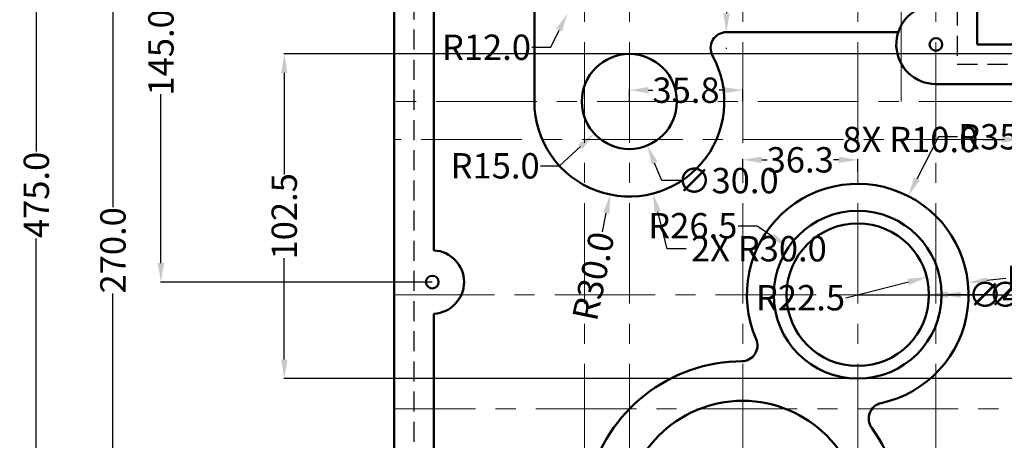
# Model space of a CAD drawing. Units: inches. Extents: x 11765 to 12471, y 10149 to 10793.
# Tile 2 of 8: x 11765 to 12076, y 10397 to 10530. Entities that reach past the tile are written whole.
import ezdxf

# ---------------------------------------------------------------- set-up
doc = ezdxf.new("R2010")
doc.units = ezdxf.units.IN
doc.header["$MEASUREMENT"] = 0
doc.linetypes.add('CENTER', pattern=[50.8, 31.75, -6.35, 6.35, -6.35])
doc.linetypes.add('HIDDEN', pattern=[9.525, 6.35, -3.175])
for name, color, linetype, lineweight in [('M-CNTR', 30, 'CENTER', 18), ('M-DIMS', 2, 'Continuous', 25), ('M-HIDN', 41, 'HIDDEN', 25), ('M-OUTL', 7, 'Continuous', 50)]:
    doc.layers.add(name, color=color, linetype=linetype, lineweight=lineweight)
doc.styles.get("Standard").update_dxf_attribs({"font": 'arial.ttf'})
doc.dimstyles.get("Standard").update_dxf_attribs({"dimtxt": 8, "dimasz": 6, "dimexe": 0.18, "dimexo": 0.0625, "dimgap": 0.09, "dimtad": 0, "dimtoh": 1, "dimdec": 1, "dimzin": 0, "dimdsep": 46, "dimtxsty": 'Standard', "dimcen": 0.09, "dimadec": 0, "dimazin": 0, "dimtfac": 1, "dimtdec": 1, "dimtofl": 0, "dimtmove": 0, "dimatfit": 3, "dimfxl": 1, "dimtolj": 1, "dimtzin": 0, "dimarcsym": 0})

# ---------------------------------------------------------------- blocks, each defined once
blk = doc.blocks.new('*D6')
at = {"layer": 'Defpoints', "color": 0, "transparency": 16777216}
for p in [(11882.91, 10712.15), (11769.87, 10237.15), (11917.55, 10237.15)]:
    blk.add_point(p, dxfattribs=at)
at = {"layer": 'M-DIMS', "color": 0, "lineweight": -2, "transparency": 16777216}
for p, q in [((11882.85, 10712.15), (11769.69, 10712.15)), ((11769.87, 10706.15), (11769.87, 10488.38)), ((11769.87, 10243.15), (11769.87, 10460.91)), ((11917.49, 10237.15), (11769.69, 10237.15))]:
    blk.add_line(p, q, dxfattribs=at)
at = {"layer": 'M-DIMS', "color": 0, "transparency": 16777216}
for points in [[(11768.87, 10706.15), (11770.87, 10706.15), (11769.87, 10712.15)], [(11768.87, 10243.15), (11770.87, 10243.15), (11769.87, 10237.15)]]:
    blk.add_solid(points, dxfattribs=at)
at = {"layer": 'M-DIMS', "color": 0, "transparency": 16777216, "insert": (11769.87, 10474.65), "char_height": 8, "attachment_point": 5, "rotation": 90}
blk.add_mtext('\\A1;475.0', dxfattribs=at)
blk = doc.blocks.new('*D12')
at = {"layer": 'Defpoints', "color": 0, "transparency": 16777216}
for p in [(12130.14, 10592.15), (12029.23, 10443.15), (12167.12, 10443.15)]:
    blk.add_point(p, dxfattribs=at)
at = {"layer": 'M-DIMS', "color": 0, "lineweight": -2, "transparency": 16777216}
for p, q in [((12130.2, 10592.15), (12167.3, 10592.15)), ((12167.12, 10586.15), (12167.12, 10530.84)), ((12167.12, 10449.15), (12167.12, 10504.45)), ((12029.29, 10443.15), (12167.3, 10443.15))]:
    blk.add_line(p, q, dxfattribs=at)
at = {"layer": 'M-DIMS', "color": 0, "transparency": 16777216}
for points in [[(12166.12, 10586.15), (12168.12, 10586.15), (12167.12, 10592.15)], [(12166.12, 10449.15), (12168.12, 10449.15), (12167.12, 10443.15)]]:
    blk.add_solid(points, dxfattribs=at)
at = {"layer": 'M-DIMS', "color": 0, "transparency": 16777216, "insert": (12167.12, 10517.65), "char_height": 8, "attachment_point": 5, "rotation": 90}
blk.add_mtext('\\A1;149.0', dxfattribs=at)
blk = doc.blocks.new('*D14')
at = {"layer": 'Defpoints', "color": 0, "transparency": 16777216}
for p in [(12156.23, 10592.15), (12216.5, 10592.15), (11992.91, 10372.15)]:
    blk.add_point(p, dxfattribs=at)
at = {"layer": 'M-DIMS', "color": 0, "lineweight": -2, "transparency": 16777216}
for p, q in [((12156.3, 10592.15), (12216.68, 10592.15)), ((12216.5, 10586.15), (12216.5, 10495.79)), ((12216.5, 10378.15), (12216.5, 10468.5)), ((11992.97, 10372.15), (12216.68, 10372.15))]:
    blk.add_line(p, q, dxfattribs=at)
at = {"layer": 'M-DIMS', "color": 0, "transparency": 16777216}
for points in [[(12215.5, 10586.15), (12217.5, 10586.15), (12216.5, 10592.15)], [(12215.5, 10378.15), (12217.5, 10378.15), (12216.5, 10372.15)]]:
    blk.add_solid(points, dxfattribs=at)
at = {"layer": 'M-DIMS', "color": 0, "transparency": 16777216, "insert": (12216.5, 10482.15), "char_height": 8, "attachment_point": 5, "rotation": 90}
blk.add_mtext('\\A1;220.0', dxfattribs=at)
blk = doc.blocks.new('*D29')
at = {"layer": 'Defpoints', "color": 0, "transparency": 16777216}
for p in [(11794.06, 10592.15), (11889.16, 10592.15), (11894.91, 10322.15)]:
    blk.add_point(p, dxfattribs=at)
at = {"layer": 'M-DIMS', "color": 0, "lineweight": -2, "transparency": 16777216}
for p, q in [((11889.1, 10592.15), (11793.88, 10592.15)), ((11794.06, 10586.15), (11794.06, 10470.79)), ((11794.06, 10328.15), (11794.06, 10443.5)), ((11894.85, 10322.15), (11793.88, 10322.15))]:
    blk.add_line(p, q, dxfattribs=at)
at = {"layer": 'M-DIMS', "color": 0, "transparency": 16777216}
for points in [[(11793.06, 10586.15), (11795.06, 10586.15), (11794.06, 10592.15)], [(11793.06, 10328.15), (11795.06, 10328.15), (11794.06, 10322.15)]]:
    blk.add_solid(points, dxfattribs=at)
at = {"layer": 'M-DIMS', "color": 0, "transparency": 16777216, "insert": (11794.06, 10457.15), "char_height": 8, "attachment_point": 5, "rotation": 90}
blk.add_mtext('\\A1;270.0', dxfattribs=at)
blk = doc.blocks.new('*D30')
at = {"layer": 'Defpoints', "color": 0, "transparency": 16777216}
for p in [(11872.35, 10592.15), (11809.21, 10447.15), (11894.91, 10447.15)]:
    blk.add_point(p, dxfattribs=at)
at = {"layer": 'M-DIMS', "color": 0, "lineweight": -2, "transparency": 16777216}
for p, q in [((11872.29, 10592.15), (11809.03, 10592.15)), ((11809.21, 10586.15), (11809.21, 10532.84)), ((11809.21, 10453.15), (11809.21, 10506.45)), ((11894.85, 10447.15), (11809.03, 10447.15))]:
    blk.add_line(p, q, dxfattribs=at)
at = {"layer": 'M-DIMS', "color": 0, "transparency": 16777216}
for points in [[(11808.21, 10586.15), (11810.21, 10586.15), (11809.21, 10592.15)], [(11808.21, 10453.15), (11810.21, 10453.15), (11809.21, 10447.15)]]:
    blk.add_solid(points, dxfattribs=at)
at = {"layer": 'M-DIMS', "color": 0, "transparency": 16777216, "insert": (11809.21, 10519.65), "char_height": 8, "attachment_point": 5, "rotation": 90}
blk.add_mtext('\\A1;145.0', dxfattribs=at)
blk = doc.blocks.new('*D37')
at = {"layer": 'Defpoints', "color": 0, "transparency": 16777216}
for p in [(11957.12, 10504.15), (11951.06, 10474.76)]:
    blk.add_point(p, dxfattribs=at)
at = {"layer": 'M-DIMS', "color": 0, "lineweight": -2, "transparency": 16777216}
for p, q in [((11957.03, 10504.15), (11957.21, 10504.15)), ((11957.12, 10504.06), (11957.12, 10504.24)), ((11948.64, 10463.01), (11949.85, 10468.89))]:
    blk.add_line(p, q, dxfattribs=at)
at = {"layer": 'M-DIMS', "color": 0, "transparency": 16777216}
blk.add_solid([(11948.87, 10469.09), (11950.83, 10468.69), (11951.06, 10474.76)], dxfattribs=at)
at = {"layer": 'M-DIMS', "color": 0, "transparency": 16777216, "insert": (11945.75, 10449.01), "char_height": 8, "attachment_point": 5, "rotation": 78.3456}
blk.add_mtext('\\A1;R30.0', dxfattribs=at)
blk = doc.blocks.new('*D38')
at = {"layer": 'Defpoints', "color": 0, "transparency": 16777216}
for p in [(11957.12, 10504.15), (11946.08, 10493.99)]:
    blk.add_point(p, dxfattribs=at)
at = {"layer": 'M-DIMS', "color": 0, "lineweight": -2, "transparency": 16777216}
for p, q in [((11957.03, 10504.15), (11957.21, 10504.15)), ((11957.12, 10504.06), (11957.12, 10504.24)), ((11935.04, 10483.84), (11941.67, 10489.93)), ((11929.04, 10483.84), (11935.04, 10483.84))]:
    blk.add_line(p, q, dxfattribs=at)
at = {"layer": 'M-DIMS', "color": 0, "transparency": 16777216}
blk.add_solid([(11940.99, 10490.66), (11942.34, 10489.19), (11946.08, 10493.99)], dxfattribs=at)
at = {"layer": 'M-DIMS', "color": 0, "transparency": 16777216, "insert": (11914.75, 10483.84), "char_height": 8, "attachment_point": 5}
blk.add_mtext('\\A1;R15.0', dxfattribs=at)
blk = doc.blocks.new('*D39')
at = {"layer": 'Defpoints', "color": 0, "transparency": 16777216}
for p in [(11942.91, 10542.79), (11937.6, 10532.03)]:
    blk.add_point(p, dxfattribs=at)
at = {"layer": 'M-DIMS', "color": 0, "lineweight": -2, "transparency": 16777216}
for p, q in [((11942.82, 10542.79), (11943, 10542.79)), ((11942.91, 10542.7), (11942.91, 10542.88)), ((11932.3, 10521.27), (11934.95, 10526.65)), ((11926.3, 10521.27), (11932.3, 10521.27))]:
    blk.add_line(p, q, dxfattribs=at)
at = {"layer": 'M-DIMS', "color": 0, "transparency": 16777216}
blk.add_solid([(11934.05, 10527.09), (11935.85, 10526.21), (11937.6, 10532.03)], dxfattribs=at)
at = {"layer": 'M-DIMS', "color": 0, "transparency": 16777216, "insert": (11912, 10521.27), "char_height": 8, "attachment_point": 5}
blk.add_mtext('\\A1;R12.0', dxfattribs=at)
blk = doc.blocks.new('*D41')
at = {"layer": 'Defpoints', "color": 0, "transparency": 16777216}
for p in [(11987.78, 10526.02), (11987.78, 10521.02)]:
    blk.add_point(p, dxfattribs=at)
at = {"layer": 'M-DIMS', "color": 0, "lineweight": -2, "transparency": 16777216}
for p, q in [((11993.78, 10538.02), (11987.78, 10538.02)), ((11987.78, 10538.02), (11987.78, 10532.02)), ((11987.69, 10521.02), (11987.87, 10521.02)), ((11987.78, 10520.93), (11987.78, 10521.11))]:
    blk.add_line(p, q, dxfattribs=at)
at = {"layer": 'M-DIMS', "color": 0, "transparency": 16777216}
blk.add_solid([(11986.78, 10532.02), (11988.78, 10532.02), (11987.78, 10526.02)], dxfattribs=at)
at = {"layer": 'M-DIMS', "color": 0, "transparency": 16777216, "insert": (12004.97, 10538.02), "char_height": 8, "attachment_point": 5}
blk.add_mtext('\\A1;R5.0', dxfattribs=at)
blk = doc.blocks.new('*D46')
at = {"layer": 'Defpoints', "color": 0, "transparency": 16777216}
for p in [(12064.02, 10446.97), (12029.23, 10443.15)]:
    blk.add_point(p, dxfattribs=at)
at = {"layer": 'M-DIMS', "color": 0, "lineweight": -2, "transparency": 16777216}
for p, q in [((12075.95, 10448.28), (12069.99, 10447.62)), ((12029.14, 10443.15), (12029.32, 10443.15)), ((12029.23, 10443.06), (12029.23, 10443.24))]:
    blk.add_line(p, q, dxfattribs=at)
at = {"layer": 'M-DIMS', "color": 0, "transparency": 16777216}
blk.add_solid([(12069.88, 10448.62), (12070.1, 10446.63), (12064.02, 10446.97)], dxfattribs=at)
at = {"layer": 'M-DIMS', "color": 0, "transparency": 16777216, "insert": (12090.25, 10448.28), "char_height": 8, "attachment_point": 5}
blk.add_mtext('\\A1;R35.0', dxfattribs=at)
blk = doc.blocks.new('*D47')
at = {"layer": 'Defpoints', "color": 0, "transparency": 16777216}
for p in [(12051.04, 10448.69), (12029.23, 10443.15)]:
    blk.add_point(p, dxfattribs=at)
at = {"layer": 'M-DIMS', "color": 0, "lineweight": -2, "transparency": 16777216}
blk.add_line((12025.51, 10442.2), (12045.22, 10447.21), dxfattribs=at)
at = {"layer": 'M-DIMS', "color": 0, "transparency": 16777216}
blk.add_solid([(12044.98, 10448.18), (12045.47, 10446.24), (12051.04, 10448.69)], dxfattribs=at)
at = {"layer": 'M-DIMS', "color": 0, "transparency": 16777216, "insert": (12011.17, 10442.2), "char_height": 8, "attachment_point": 5}
blk.add_mtext('\\A1;R22.5', dxfattribs=at)
blk = doc.blocks.new('*D48')
at = {"layer": 'Defpoints', "color": 0, "transparency": 16777216}
for p in [(12007.38, 10458.14), (12029.23, 10443.15)]:
    blk.add_point(p, dxfattribs=at)
at = {"layer": 'M-DIMS', "color": 0, "lineweight": -2, "transparency": 16777216}
for p, q in [((11991.49, 10464.93), (11997.49, 10464.93)), ((11997.49, 10464.93), (12002.43, 10461.53)), ((12029.14, 10443.15), (12029.32, 10443.15)), ((12029.23, 10443.06), (12029.23, 10443.24))]:
    blk.add_line(p, q, dxfattribs=at)
at = {"layer": 'M-DIMS', "color": 0, "transparency": 16777216}
blk.add_solid([(12003, 10462.36), (12001.87, 10460.71), (12007.38, 10458.14)], dxfattribs=at)
at = {"layer": 'M-DIMS', "color": 0, "transparency": 16777216, "insert": (11977.15, 10464.93), "char_height": 8, "attachment_point": 5}
blk.add_mtext('\\A1;R26.5', dxfattribs=at)
blk = doc.blocks.new('*D51')
at = {"layer": 'Defpoints', "color": 0, "transparency": 16777216}
for p in [(12029.23, 10485.73), (11992.91, 10481.96), (12029.23, 10481.96)]:
    blk.add_point(p, dxfattribs=at)
at = {"layer": 'M-DIMS', "color": 0, "lineweight": -2, "transparency": 16777216}
for p, q in [((11992.91, 10482.03), (11992.91, 10485.91)), ((11998.91, 10485.73), (12000.59, 10485.73)), ((12023.23, 10485.73), (12021.55, 10485.73)), ((12029.23, 10482.03), (12029.23, 10485.91))]:
    blk.add_line(p, q, dxfattribs=at)
at = {"layer": 'M-DIMS', "color": 0, "transparency": 16777216}
for points in [[(11998.91, 10486.73), (11998.91, 10484.73), (11992.91, 10485.73)], [(12023.23, 10486.73), (12023.23, 10484.73), (12029.23, 10485.73)]]:
    blk.add_solid(points, dxfattribs=at)
at = {"layer": 'M-DIMS', "color": 0, "transparency": 16777216, "insert": (12011.07, 10485.73), "char_height": 8, "attachment_point": 5}
blk.add_mtext('\\A1;36.3', dxfattribs=at)
blk = doc.blocks.new('*D52')
at = {"layer": 'Defpoints', "color": 0, "transparency": 16777216}
for p in [(11992.91, 10507.72), (11957.12, 10504.15), (11992.91, 10504.24)]:
    blk.add_point(p, dxfattribs=at)
at = {"layer": 'M-DIMS', "color": 0, "lineweight": -2, "transparency": 16777216}
for p, q in [((11957.12, 10504.21), (11957.12, 10507.9)), ((11963.12, 10507.72), (11964.53, 10507.72)), ((11986.91, 10507.72), (11985.5, 10507.72)), ((11992.91, 10504.3), (11992.91, 10507.9))]:
    blk.add_line(p, q, dxfattribs=at)
at = {"layer": 'M-DIMS', "color": 0, "transparency": 16777216}
for points in [[(11963.12, 10508.72), (11963.12, 10506.72), (11957.12, 10507.72)], [(11986.91, 10508.72), (11986.91, 10506.72), (11992.91, 10507.72)]]:
    blk.add_solid(points, dxfattribs=at)
at = {"layer": 'M-DIMS', "color": 0, "transparency": 16777216, "insert": (11975.02, 10507.72), "char_height": 8, "attachment_point": 5}
blk.add_mtext('\\A1;35.8', dxfattribs=at)
blk = doc.blocks.new('*D66')
at = {"layer": 'Defpoints', "color": 0, "transparency": 16777216}
for p in [(12386.9, 10519.15), (11848.16, 10416.65), (12386.9, 10416.65)]:
    blk.add_point(p, dxfattribs=at)
at = {"layer": 'M-DIMS', "color": 0, "lineweight": -2, "transparency": 16777216}
for p, q in [((12386.83, 10519.15), (11847.98, 10519.15)), ((11848.16, 10513.15), (11848.16, 10481.14)), ((11848.16, 10422.65), (11848.16, 10454.65)), ((12386.83, 10416.65), (11847.98, 10416.65))]:
    blk.add_line(p, q, dxfattribs=at)
at = {"layer": 'M-DIMS', "color": 0, "transparency": 16777216}
for points in [[(11847.16, 10513.15), (11849.16, 10513.15), (11848.16, 10519.15)], [(11847.16, 10422.65), (11849.16, 10422.65), (11848.16, 10416.65)]]:
    blk.add_solid(points, dxfattribs=at)
at = {"layer": 'M-DIMS', "color": 0, "transparency": 16777216, "insert": (11848.16, 10467.9), "char_height": 8, "attachment_point": 5, "rotation": 90}
blk.add_mtext('\\A1;102.5', dxfattribs=at)
blk = doc.blocks.new('*D71')
at = {"layer": 'Defpoints', "color": 0, "transparency": 16777216}
for p in [(12045.17, 10474.31), (12029.23, 10443.15)]:
    blk.add_point(p, dxfattribs=at)
at = {"layer": 'M-DIMS', "color": 0, "lineweight": -2, "transparency": 16777216}
for p, q in [((12054.74, 10493), (12047.9, 10479.65)), ((12060.74, 10493), (12054.74, 10493)), ((12029.14, 10443.15), (12029.32, 10443.15)), ((12029.23, 10443.06), (12029.23, 10443.24))]:
    blk.add_line(p, q, dxfattribs=at)
at = {"layer": 'M-DIMS', "color": 0, "transparency": 16777216}
blk.add_solid([(12047.01, 10480.1), (12048.79, 10479.19), (12045.17, 10474.31)], dxfattribs=at)
at = {"layer": 'M-DIMS', "color": 0, "transparency": 16777216, "insert": (12075.03, 10493), "char_height": 8, "attachment_point": 5}
blk.add_mtext('\\A1;R35.0', dxfattribs=at)
blk = doc.blocks.new('*D72')
at = {"layer": 'Defpoints', "color": 0, "transparency": 16777216}
for p in [(11957.12, 10504.15), (11964.59, 10475.09)]:
    blk.add_point(p, dxfattribs=at)
at = {"layer": 'M-DIMS', "color": 0, "lineweight": -2, "transparency": 16777216}
for p, q in [((11957.03, 10504.15), (11957.21, 10504.15)), ((11957.12, 10504.06), (11957.12, 10504.24)), ((11969.07, 10457.66), (11966.08, 10469.28)), ((11975.07, 10457.66), (11969.07, 10457.66))]:
    blk.add_line(p, q, dxfattribs=at)
at = {"layer": 'M-DIMS', "color": 0, "transparency": 16777216}
blk.add_solid([(11967.05, 10469.53), (11965.12, 10469.03), (11964.59, 10475.09)], dxfattribs=at)
at = {"layer": 'M-DIMS', "color": 0, "transparency": 16777216, "insert": (11998.03, 10457.66), "char_height": 8, "attachment_point": 5}
blk.add_mtext('\\A1;2X R30.0', dxfattribs=at)
blk = doc.blocks.new('*D73')
at = {"layer": 'Defpoints', "color": 0, "transparency": 16777216}
for p in [(12002.73, 10443.15), (12055.73, 10443.15)]:
    blk.add_point(p, dxfattribs=at)
at = {"layer": 'M-DIMS', "color": 0, "lineweight": -2, "transparency": 16777216}
for p, q in [((12029.14, 10443.15), (12029.32, 10443.15)), ((12029.23, 10443.06), (12029.23, 10443.24)), ((12071.63, 10443.15), (12061.73, 10443.15))]:
    blk.add_line(p, q, dxfattribs=at)
at = {"layer": 'M-DIMS', "color": 0, "transparency": 16777216}
blk.add_solid([(12061.73, 10444.15), (12061.73, 10442.15), (12055.73, 10443.15)], dxfattribs=at)
at = {"layer": 'M-DIMS', "color": 0, "transparency": 16777216, "insert": (12086.45, 10443.15), "char_height": 8, "attachment_point": 5}
blk.add_mtext('\\A1;∅53.0', dxfattribs=at)
blk = doc.blocks.new('*D74')
at = {"layer": 'Defpoints', "color": 0, "transparency": 16777216}
for p in [(12006.73, 10443.15), (12051.73, 10443.15)]:
    blk.add_point(p, dxfattribs=at)
at = {"layer": 'M-DIMS', "color": 0, "lineweight": -2, "transparency": 16777216}
for p, q in [((12029.14, 10443.15), (12029.32, 10443.15)), ((12029.23, 10443.06), (12029.23, 10443.24)), ((12065.23, 10443.15), (12057.73, 10443.15))]:
    blk.add_line(p, q, dxfattribs=at)
at = {"layer": 'M-DIMS', "color": 0, "transparency": 16777216}
blk.add_solid([(12057.73, 10444.15), (12057.73, 10442.15), (12051.73, 10443.15)], dxfattribs=at)
at = {"layer": 'M-DIMS', "color": 0, "transparency": 16777216, "insert": (12080.05, 10443.15), "char_height": 8, "attachment_point": 5}
blk.add_mtext('\\A1;∅45.0', dxfattribs=at)
blk = doc.blocks.new('*D75')
at = {"layer": 'Defpoints', "color": 0, "transparency": 16777216}
for p in [(11951.42, 10518.02), (11962.83, 10490.27)]:
    blk.add_point(p, dxfattribs=at)
at = {"layer": 'M-DIMS', "color": 0, "lineweight": -2, "transparency": 16777216}
for p, q in [((11957.03, 10504.15), (11957.21, 10504.15)), ((11957.12, 10504.06), (11957.12, 10504.24)), ((11967.39, 10479.17), (11965.11, 10484.72)), ((11973.39, 10479.17), (11967.39, 10479.17))]:
    blk.add_line(p, q, dxfattribs=at)
at = {"layer": 'M-DIMS', "color": 0, "transparency": 16777216}
blk.add_solid([(11966.03, 10485.1), (11964.18, 10484.34), (11962.83, 10490.27)], dxfattribs=at)
at = {"layer": 'M-DIMS', "color": 0, "transparency": 16777216, "insert": (11988.21, 10479.17), "char_height": 8, "attachment_point": 5}
blk.add_mtext('\\A1;∅30.0', dxfattribs=at)
blk = doc.blocks.new('*D79')
at = {"layer": 'Defpoints', "color": 0, "transparency": 16777216}
for p in [(12080.75, 10492.15), (12090.75, 10492.15)]:
    blk.add_point(p, dxfattribs=at)
at = {"layer": 'M-DIMS', "color": 0, "lineweight": -2, "transparency": 16777216}
for p, q in [((12068.75, 10492.15), (12074.75, 10492.15)), ((12090.66, 10492.15), (12090.84, 10492.15)), ((12090.75, 10492.06), (12090.75, 10492.24))]:
    blk.add_line(p, q, dxfattribs=at)
at = {"layer": 'M-DIMS', "color": 0, "transparency": 16777216}
blk.add_solid([(12074.75, 10493.15), (12074.75, 10491.15), (12080.75, 10492.15)], dxfattribs=at)
at = {"layer": 'M-DIMS', "color": 0, "transparency": 16777216, "insert": (12045.85, 10492.15), "char_height": 8, "attachment_point": 5}
blk.add_mtext('\\A1;8X R10.0', dxfattribs=at)

msp = doc.modelspace()

# ---------------------------------------------------------------- linework, layer by layer
at = {"layer": 'M-CNTR'}
for p, q in [((11942.912, 10237.146), (11942.912, 10712.146)), ((11957.122, 10237.146), (11957.122, 10712.146)), ((11992.912, 10237.146), (11992.912, 10712.146)), ((12029.232, 10237.146), (12029.232, 10712.146)), ((12042.912, 10504.146), (12042.912, 10712.146)), ((12053.912, 10237.146), (12053.912, 10712.146)), ((12131.07, 10504.146), (11882.912, 10504.146)), ((12227.966, 10492.146), (11882.912, 10492.146)), ((12066.912, 10443.146), (11882.912, 10443.146)), ((12213.332, 10407.146), (11882.912, 10407.146))]:
    msp.add_line(p, q, dxfattribs=at)
at = {"layer": 'M-HIDN'}
msp.add_lwpolyline([(12060.662, 10705.896), (12060.662, 10515.896), (12096.662, 10515.896), (12096.662, 10263.352), (12062.096, 10243.396), (11923.728, 10243.396), (11889.162, 10263.352), (11889.162, 10705.896)], close=True, dxfattribs=at)
at = {"layer": 'M-OUTL'}
for p, q in [((11882.912, 10712.146), (11882.912, 10257.146)), ((12066.912, 10522.146), (12066.912, 10712.146)), ((11927.122, 10504.146), (11927.122, 10621.706)), ((11895.412, 10562.158), (11895.412, 10457.133)), ((11987.783, 10526.025), (12042.029, 10526.025)), ((12102.912, 10522.146), (12066.912, 10522.146)), ((12089.912, 10509.646), (12053.912, 10509.646)), ((11895.412, 10437.158), (11895.412, 10332.133))]:
    msp.add_line(p, q, dxfattribs=at)
for centre, radius in [((12053.912, 10522.146), 2), ((11957.122, 10504.146), 15), ((12029.232, 10443.146), 26.5), ((12029.232, 10443.146), 22.5), ((11894.912, 10447.146), 2), ((11992.912, 10372.146), 37.5)]:
    msp.add_circle(centre, radius, dxfattribs=at)
for centre, radius, start, end in [((12053.912, 10522.146), 12.5, 94.58857, 270), ((11987.783, 10521.025), 5, 90, 208.83315), ((11957.122, 10504.146), 30, 180, 28.83315), ((12029.232, 10443.146), 35, 282.23621, 203.57982), ((11894.912, 10447.146), 10, 272.86598, 87.13402), ((11992.572, 10427.145), 5, 270.35435, 23.57982), ((11992.912, 10372.146), 50, 90, 35.46169), ((12037.71, 10404.054), 5, 102.23621, 215.46169)]:
    msp.add_arc(centre, radius, start, end, dxfattribs=at)

# ---------------------------------------------------------------- dimensions: what is measured, and where the dimension line sits
at = {"layer": 'M-DIMS'}
for base, p1, p2, override, picture, middle in [((11769.869, 10237.146), (11882.912, 10712.146), (11917.553, 10237.146), {"dimclrd": 0, "dimclre": 0, "dimclrt": 0}, '*D6', (11769.869, 10474.646)), ((11794.063, 10592.146), (11894.912, 10322.146), (11889.162, 10592.146), {"dimclrd": 0, "dimclre": 0, "dimclrt": 0}, '*D29', (11794.063, 10457.146)), ((11809.207, 10447.146), (11872.348, 10592.146), (11894.912, 10447.146), {"dimclrd": 0, "dimclre": 0, "dimclrt": 0}, '*D30', (11809.207, 10519.646)), ((12216.505, 10592.146), (11992.912, 10372.146), (12156.234, 10592.146), {"dimclrd": 0, "dimclre": 0, "dimclrt": 0}, '*D14', (12216.505, 10482.146)), ((12167.122, 10443.146), (12130.138, 10592.146), (12029.232, 10443.146), {"dimclrd": 0, "dimclre": 0, "dimclrt": 0}, '*D12', (12167.122, 10517.646)), ((11848.162, 10416.646), (12386.896, 10519.146), (12386.896, 10416.646), {"dimdec": 1, "dimlfac": 1, "dimrnd": 0, "dimzin": 0, "dimdsep": 46, "dimlunit": 2}, '*D66', (11848.162, 10467.896))]:
    dim = msp.add_linear_dim(base=base, p1=p1, p2=p2, angle=90, dimstyle='Standard', override=override, dxfattribs=at)
    dim.commit()
    dim.dimension.update_dxf_attribs({"geometry": picture, "text_midpoint": middle})
for center, mpoint, picture, middle in [((11942.912, 10542.793), (11937.604, 10532.031), '*D39', (11912.001, 10521.268)), ((11987.783, 10521.025), (11987.783, 10526.025), '*D41', (12004.97, 10538.025)), ((11957.122, 10504.146), (11951.062, 10474.764), '*D37', (11945.75, 10449.011)), ((12029.232, 10443.146), (12007.381, 10458.139), '*D48', (11977.148, 10464.928)), ((12029.232, 10443.146), (12064.023, 10446.969), '*D46', (12090.245, 10448.28))]:
    dim = msp.add_radius_dim(center=center, mpoint=mpoint, dimstyle='Standard', override={"dimclrd": 0, "dimclre": 0, "dimclrt": 0}, dxfattribs=at)
    dim.commit()
    dim.dimension.update_dxf_attribs({"geometry": picture, "text_midpoint": middle})
dim = msp.add_diameter_dim_2p(p1=(11951.417, 10518.018), p2=(11962.827, 10490.273), dimstyle='Standard', override={"dimdec": 1, "dimlfac": 1, "dimrnd": 0, "dimzin": 0, "dimdsep": 46, "dimlunit": 2}, dxfattribs=at)
dim.commit()
dim.dimension.update_dxf_attribs({"geometry": '*D75', "text_midpoint": (11988.21, 10479.175)})
for base, p1, p2, picture, middle in [((11992.912, 10507.721), (11957.122, 10504.146), (11992.912, 10504.236), '*D52', (11975.017, 10507.721)), ((12029.232, 10485.728), (11992.912, 10481.965), (12029.232, 10481.965), '*D51', (12011.072, 10485.728))]:
    dim = msp.add_linear_dim(base=base, p1=p1, p2=p2, dimstyle='Standard', override={"dimclrd": 0, "dimclre": 0, "dimclrt": 0}, dxfattribs=at)
    dim.commit()
    dim.dimension.update_dxf_attribs({"geometry": picture, "text_midpoint": middle})
for center, mpoint, override, picture, middle in [((11957.122, 10504.146), (11946.082, 10493.99), {"dimclrd": 0, "dimclre": 0, "dimclrt": 0}, '*D38', (11914.748, 10483.835)), ((12029.232, 10443.146), (12045.172, 10474.305), {"dimdec": 1, "dimlfac": 1, "dimrnd": 0, "dimzin": 0, "dimdsep": 46, "dimlunit": 2}, '*D71', (12075.031, 10493.001)), ((12029.232, 10443.146), (12051.039, 10448.686), {"dimclrd": 0, "dimclre": 0, "dimclrt": 0}, '*D47', (12025.512, 10442.2))]:
    dim = msp.add_radius_dim(center=center, mpoint=mpoint, dimstyle='Standard', override=override, dxfattribs=at)
    dim.commit()
    dim.dimension.update_dxf_attribs({"geometry": picture, "text_midpoint": middle, "dimtype": 164})
dim = msp.add_radius_dim(center=(11957.122, 10504.146), mpoint=(11964.591, 10475.09), text='2X <>', dimstyle='Standard', override={"dimdec": 1, "dimlfac": 1, "dimrnd": 0, "dimzin": 0, "dimdsep": 46, "dimlunit": 2}, dxfattribs=at)
dim.commit()
dim.dimension.update_dxf_attribs({"geometry": '*D72', "text_midpoint": (11998.03, 10457.657), "dimtype": 164})
dim = msp.add_radius_dim(center=(12090.748, 10492.146), mpoint=(12080.748, 10492.15), text='8X <>', dimstyle='Standard', override={"dimdec": 1, "dimlfac": 1, "dimrnd": 0, "dimzin": 0, "dimdsep": 46, "dimlunit": 2}, dxfattribs=at)
dim.commit()
dim.dimension.update_dxf_attribs({"geometry": '*D79', "text_midpoint": (12045.853, 10492.155)})
for p1, p2, picture, middle in [((12002.732, 10443.145), (12055.732, 10443.146), '*D73', (12071.632, 10443.146)), ((12006.732, 10443.145), (12051.732, 10443.146), '*D74', (12065.232, 10443.146))]:
    dim = msp.add_diameter_dim_2p(p1=p1, p2=p2, dimstyle='Standard', override={"dimdec": 1, "dimlfac": 1, "dimrnd": 0, "dimzin": 0, "dimdsep": 46, "dimlunit": 2}, dxfattribs=at)
    dim.commit()
    dim.dimension.update_dxf_attribs({"geometry": picture, "text_midpoint": middle, "dimtype": 163})

doc.saveas('drawing.dxf')
